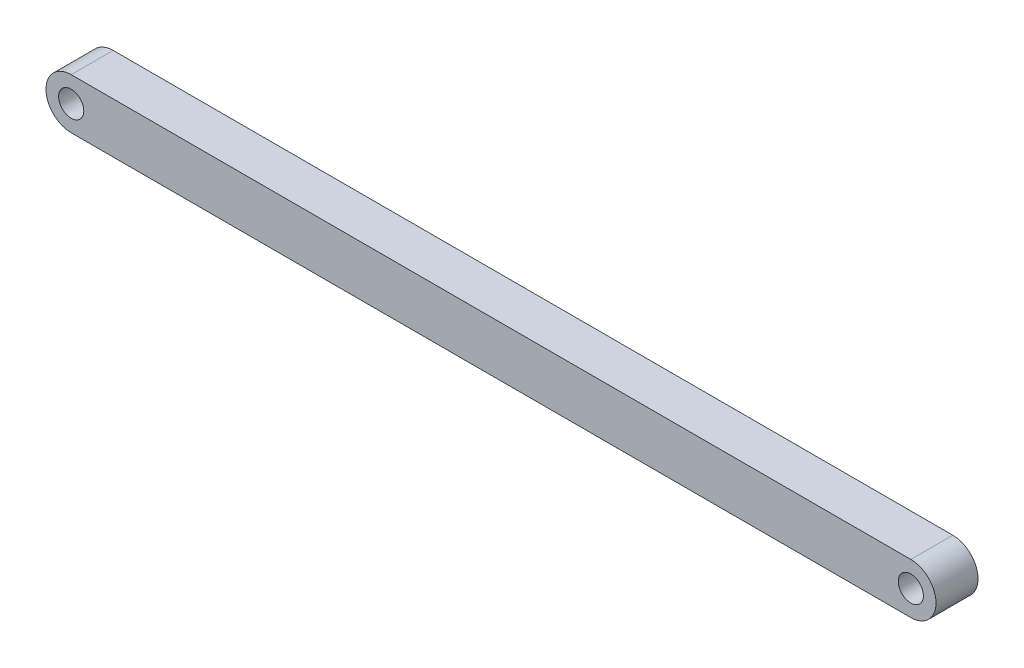
ISO-10303-21;
HEADER;
FILE_DESCRIPTION(('STEP AP214'),'2;1');
FILE_NAME('part.step','',(''),(''),'','','');
FILE_SCHEMA(('AUTOMOTIVE_DESIGN { 1 0 10303 214 1 1 1 1 }'));
ENDSEC;
DATA;
#1=APPLICATION_CONTEXT('core data for automotive mechanical design processes');
#2=APPLICATION_PROTOCOL_DEFINITION('international standard','automotive_design',2000,#1);
#3=PRODUCT_CONTEXT('',#1,'mechanical');
#4=PRODUCT('Part','Part','',(#3));
#5=PRODUCT_RELATED_PRODUCT_CATEGORY('part','',(#4));
#6=PRODUCT_DEFINITION_FORMATION('','',#4);
#7=PRODUCT_DEFINITION_CONTEXT('part definition',#1,'design');
#8=PRODUCT_DEFINITION('design','',#6,#7);
#9=PRODUCT_DEFINITION_SHAPE('','',#8);
#10=(LENGTH_UNIT() NAMED_UNIT(*) SI_UNIT(.MILLI.,.METRE.));
#11=(NAMED_UNIT(*) PLANE_ANGLE_UNIT() SI_UNIT($,.RADIAN.));
#12=(NAMED_UNIT(*) SI_UNIT($,.STERADIAN.) SOLID_ANGLE_UNIT());
#13=UNCERTAINTY_MEASURE_WITH_UNIT(LENGTH_MEASURE(1.E-05),#10,'distance_accuracy_value','');
#14=(GEOMETRIC_REPRESENTATION_CONTEXT(3) GLOBAL_UNCERTAINTY_ASSIGNED_CONTEXT((#13)) GLOBAL_UNIT_ASSIGNED_CONTEXT((#10,
#11,#12)) REPRESENTATION_CONTEXT('',''));
#15=CARTESIAN_POINT('',(0.,0.,0.));
#16=DIRECTION('',(0.,0.,1.));
#17=DIRECTION('',(1.,0.,0.));
#18=AXIS2_PLACEMENT_3D('',#15,#16,#17);
#19=CARTESIAN_POINT('',(-50.,0.,5.));
#20=DIRECTION('',(0.,0.,1.));
#21=DIRECTION('',(1.,0.,0.));
#22=AXIS2_PLACEMENT_3D('',#19,#20,#21);
#23=PLANE('',#22);
#24=CARTESIAN_POINT('',(-50.,0.,5.));
#25=DIRECTION('',(0.,0.,1.));
#26=DIRECTION('',(1.,0.,0.));
#27=AXIS2_PLACEMENT_3D('',#24,#25,#26);
#28=CIRCLE('',#27,1.5);
#29=CARTESIAN_POINT('',(-48.5,0.,5.));
#30=VERTEX_POINT('',#29);
#31=EDGE_CURVE('E106',#30,#30,#28,.T.);
#32=ORIENTED_EDGE('',*,*,#31,.F.);
#33=EDGE_LOOP('',(#32));
#34=FACE_BOUND('',#33,.T.);
#35=CARTESIAN_POINT('',(-50.,0.,5.));
#36=DIRECTION('',(0.,0.,1.));
#37=DIRECTION('',(1.,0.,0.));
#38=AXIS2_PLACEMENT_3D('',#35,#36,#37);
#39=CIRCLE('',#38,3.00000000000002);
#40=CARTESIAN_POINT('',(-50.,3.00000000000002,5.));
#41=VERTEX_POINT('',#40);
#42=CARTESIAN_POINT('',(-50.,-3.00000000000002,5.));
#43=VERTEX_POINT('',#42);
#44=EDGE_CURVE('E93',#41,#43,#39,.T.);
#45=ORIENTED_EDGE('',*,*,#44,.T.);
#46=DIRECTION('',(1.,0.,0.));
#47=VECTOR('',#46,1.);
#48=CARTESIAN_POINT('',(-50.,-3.00000000000002,5.));
#49=LINE('',#48,#47);
#50=CARTESIAN_POINT('',(50.,-3.00000000000002,5.));
#51=VERTEX_POINT('',#50);
#52=EDGE_CURVE('E88',#43,#51,#49,.T.);
#53=ORIENTED_EDGE('',*,*,#52,.T.);
#54=CARTESIAN_POINT('',(50.,0.,5.));
#55=DIRECTION('',(0.,0.,1.));
#56=DIRECTION('',(1.,0.,0.));
#57=AXIS2_PLACEMENT_3D('',#54,#55,#56);
#58=CIRCLE('',#57,3.00000000000002);
#59=CARTESIAN_POINT('',(50.,3.00000000000004,5.));
#60=VERTEX_POINT('',#59);
#61=EDGE_CURVE('E90',#51,#60,#58,.T.);
#62=ORIENTED_EDGE('',*,*,#61,.T.);
#63=DIRECTION('',(-1.,0.,0.));
#64=VECTOR('',#63,1.);
#65=CARTESIAN_POINT('',(-50.,3.00000000000002,5.));
#66=LINE('',#65,#64);
#67=EDGE_CURVE('E57',#60,#41,#66,.T.);
#68=ORIENTED_EDGE('',*,*,#67,.T.);
#69=EDGE_LOOP('',(#45,#53,#62,#68));
#70=FACE_BOUND('',#69,.T.);
#71=CARTESIAN_POINT('',(50.,0.,5.));
#72=DIRECTION('',(0.,0.,1.));
#73=DIRECTION('',(1.,0.,0.));
#74=AXIS2_PLACEMENT_3D('',#71,#72,#73);
#75=CIRCLE('',#74,1.5);
#76=CARTESIAN_POINT('',(51.5,0.,5.));
#77=VERTEX_POINT('',#76);
#78=EDGE_CURVE('E124',#77,#77,#75,.T.);
#79=ORIENTED_EDGE('',*,*,#78,.F.);
#80=EDGE_LOOP('',(#79));
#81=FACE_BOUND('',#80,.T.);
#82=ADVANCED_FACE('F39',(#34,#70,#81),#23,.T.);
#83=CARTESIAN_POINT('',(-50.,0.,0.));
#84=DIRECTION('',(0.,0.,1.));
#85=DIRECTION('',(1.,0.,0.));
#86=AXIS2_PLACEMENT_3D('',#83,#84,#85);
#87=PLANE('',#86);
#88=CARTESIAN_POINT('',(-50.,0.,0.));
#89=DIRECTION('',(0.,0.,1.));
#90=DIRECTION('',(1.,0.,0.));
#91=AXIS2_PLACEMENT_3D('',#88,#89,#90);
#92=CIRCLE('',#91,3.00000000000002);
#93=CARTESIAN_POINT('',(-50.,3.00000000000002,0.));
#94=VERTEX_POINT('',#93);
#95=CARTESIAN_POINT('',(-50.,-3.00000000000002,0.));
#96=VERTEX_POINT('',#95);
#97=EDGE_CURVE('E103',#94,#96,#92,.T.);
#98=ORIENTED_EDGE('',*,*,#97,.F.);
#99=DIRECTION('',(-1.,0.,0.));
#100=VECTOR('',#99,1.);
#101=CARTESIAN_POINT('',(-50.,3.00000000000002,0.));
#102=LINE('',#101,#100);
#103=CARTESIAN_POINT('',(50.,3.00000000000004,0.));
#104=VERTEX_POINT('',#103);
#105=EDGE_CURVE('E76',#104,#94,#102,.T.);
#106=ORIENTED_EDGE('',*,*,#105,.F.);
#107=CARTESIAN_POINT('',(50.,0.,0.));
#108=DIRECTION('',(0.,0.,1.));
#109=DIRECTION('',(1.,0.,0.));
#110=AXIS2_PLACEMENT_3D('',#107,#108,#109);
#111=CIRCLE('',#110,3.00000000000002);
#112=CARTESIAN_POINT('',(50.,-3.00000000000002,0.));
#113=VERTEX_POINT('',#112);
#114=EDGE_CURVE('E71',#113,#104,#111,.T.);
#115=ORIENTED_EDGE('',*,*,#114,.F.);
#116=DIRECTION('',(1.,0.,0.));
#117=VECTOR('',#116,1.);
#118=CARTESIAN_POINT('',(-50.,-3.00000000000002,0.));
#119=LINE('',#118,#117);
#120=EDGE_CURVE('E92',#96,#113,#119,.T.);
#121=ORIENTED_EDGE('',*,*,#120,.F.);
#122=EDGE_LOOP('',(#98,#106,#115,#121));
#123=FACE_BOUND('',#122,.T.);
#124=CARTESIAN_POINT('',(-50.,0.,0.));
#125=DIRECTION('',(0.,0.,1.));
#126=DIRECTION('',(1.,0.,0.));
#127=AXIS2_PLACEMENT_3D('',#124,#125,#126);
#128=CIRCLE('',#127,1.5);
#129=CARTESIAN_POINT('',(-48.5,0.,0.));
#130=VERTEX_POINT('',#129);
#131=EDGE_CURVE('E119',#130,#130,#128,.T.);
#132=ORIENTED_EDGE('',*,*,#131,.T.);
#133=EDGE_LOOP('',(#132));
#134=FACE_BOUND('',#133,.T.);
#135=CARTESIAN_POINT('',(50.,0.,0.));
#136=DIRECTION('',(0.,0.,1.));
#137=DIRECTION('',(1.,0.,0.));
#138=AXIS2_PLACEMENT_3D('',#135,#136,#137);
#139=CIRCLE('',#138,1.5);
#140=CARTESIAN_POINT('',(51.5,0.,0.));
#141=VERTEX_POINT('',#140);
#142=EDGE_CURVE('E123',#141,#141,#139,.T.);
#143=ORIENTED_EDGE('',*,*,#142,.T.);
#144=EDGE_LOOP('',(#143));
#145=FACE_BOUND('',#144,.T.);
#146=ADVANCED_FACE('F111',(#123,#134,#145),#87,.F.);
#147=CARTESIAN_POINT('',(-50.,0.,5.));
#148=DIRECTION('',(0.,0.,-1.));
#149=DIRECTION('',(-1.,0.,0.));
#150=AXIS2_PLACEMENT_3D('',#147,#148,#149);
#151=CYLINDRICAL_SURFACE('',#150,3.00000000000002);
#152=ORIENTED_EDGE('',*,*,#97,.T.);
#153=DIRECTION('',(0.,0.,-1.));
#154=VECTOR('',#153,1.);
#155=CARTESIAN_POINT('',(-50.,-3.00000000000002,5.));
#156=LINE('',#155,#154);
#157=EDGE_CURVE('E11',#43,#96,#156,.T.);
#158=ORIENTED_EDGE('',*,*,#157,.F.);
#159=ORIENTED_EDGE('',*,*,#44,.F.);
#160=DIRECTION('',(0.,0.,-1.));
#161=VECTOR('',#160,1.);
#162=CARTESIAN_POINT('',(-50.,3.00000000000002,5.));
#163=LINE('',#162,#161);
#164=EDGE_CURVE('E97',#41,#94,#163,.T.);
#165=ORIENTED_EDGE('',*,*,#164,.T.);
#166=EDGE_LOOP('',(#152,#158,#159,#165));
#167=FACE_BOUND('',#166,.T.);
#168=ADVANCED_FACE('F41',(#167),#151,.T.);
#169=CARTESIAN_POINT('',(-50.,-3.00000000000002,5.));
#170=DIRECTION('',(0.,1.,0.));
#171=DIRECTION('',(-1.,0.,0.));
#172=AXIS2_PLACEMENT_3D('',#169,#170,#171);
#173=PLANE('',#172);
#174=ORIENTED_EDGE('',*,*,#120,.T.);
#175=DIRECTION('',(0.,0.,-1.));
#176=VECTOR('',#175,1.);
#177=CARTESIAN_POINT('',(50.,-3.00000000000002,5.));
#178=LINE('',#177,#176);
#179=EDGE_CURVE('E48',#51,#113,#178,.T.);
#180=ORIENTED_EDGE('',*,*,#179,.F.);
#181=ORIENTED_EDGE('',*,*,#52,.F.);
#182=ORIENTED_EDGE('',*,*,#157,.T.);
#183=EDGE_LOOP('',(#174,#180,#181,#182));
#184=FACE_BOUND('',#183,.T.);
#185=ADVANCED_FACE('F94',(#184),#173,.F.);
#186=CARTESIAN_POINT('',(50.,0.,5.));
#187=DIRECTION('',(0.,0.,-1.));
#188=DIRECTION('',(-1.,0.,0.));
#189=AXIS2_PLACEMENT_3D('',#186,#187,#188);
#190=CYLINDRICAL_SURFACE('',#189,3.00000000000002);
#191=ORIENTED_EDGE('',*,*,#114,.T.);
#192=DIRECTION('',(0.,0.,-1.));
#193=VECTOR('',#192,1.);
#194=CARTESIAN_POINT('',(50.,3.00000000000004,5.));
#195=LINE('',#194,#193);
#196=EDGE_CURVE('E96',#60,#104,#195,.T.);
#197=ORIENTED_EDGE('',*,*,#196,.F.);
#198=ORIENTED_EDGE('',*,*,#61,.F.);
#199=ORIENTED_EDGE('',*,*,#179,.T.);
#200=EDGE_LOOP('',(#191,#197,#198,#199));
#201=FACE_BOUND('',#200,.T.);
#202=ADVANCED_FACE('F100',(#201),#190,.T.);
#203=CARTESIAN_POINT('',(-50.,3.00000000000002,5.));
#204=DIRECTION('',(0.,-1.,0.));
#205=DIRECTION('',(1.,0.,0.));
#206=AXIS2_PLACEMENT_3D('',#203,#204,#205);
#207=PLANE('',#206);
#208=ORIENTED_EDGE('',*,*,#105,.T.);
#209=ORIENTED_EDGE('',*,*,#164,.F.);
#210=ORIENTED_EDGE('',*,*,#67,.F.);
#211=ORIENTED_EDGE('',*,*,#196,.T.);
#212=EDGE_LOOP('',(#208,#209,#210,#211));
#213=FACE_BOUND('',#212,.T.);
#214=ADVANCED_FACE('F112',(#213),#207,.F.);
#215=CARTESIAN_POINT('',(-50.,0.,5.));
#216=DIRECTION('',(0.,0.,-1.));
#217=DIRECTION('',(-1.,0.,0.));
#218=AXIS2_PLACEMENT_3D('',#215,#216,#217);
#219=CYLINDRICAL_SURFACE('',#218,1.5);
#220=ORIENTED_EDGE('',*,*,#31,.T.);
#221=EDGE_LOOP('',(#220));
#222=FACE_BOUND('',#221,.T.);
#223=ORIENTED_EDGE('',*,*,#131,.F.);
#224=EDGE_LOOP('',(#223));
#225=FACE_BOUND('',#224,.T.);
#226=ADVANCED_FACE('F143',(#222,#225),#219,.F.);
#227=CARTESIAN_POINT('',(50.,0.,5.));
#228=DIRECTION('',(0.,0.,-1.));
#229=DIRECTION('',(-1.,0.,0.));
#230=AXIS2_PLACEMENT_3D('',#227,#228,#229);
#231=CYLINDRICAL_SURFACE('',#230,1.5);
#232=ORIENTED_EDGE('',*,*,#78,.T.);
#233=EDGE_LOOP('',(#232));
#234=FACE_BOUND('',#233,.T.);
#235=ORIENTED_EDGE('',*,*,#142,.F.);
#236=EDGE_LOOP('',(#235));
#237=FACE_BOUND('',#236,.T.);
#238=ADVANCED_FACE('F128',(#234,#237),#231,.F.);
#239=CLOSED_SHELL('',(#82,#146,#168,#185,#202,#214,#226,#238));
#240=MANIFOLD_SOLID_BREP('B2',#239);
#241=ADVANCED_BREP_SHAPE_REPRESENTATION('',(#18,#240),#14);
#242=SHAPE_DEFINITION_REPRESENTATION(#9,#241);
ENDSEC;
END-ISO-10303-21;
